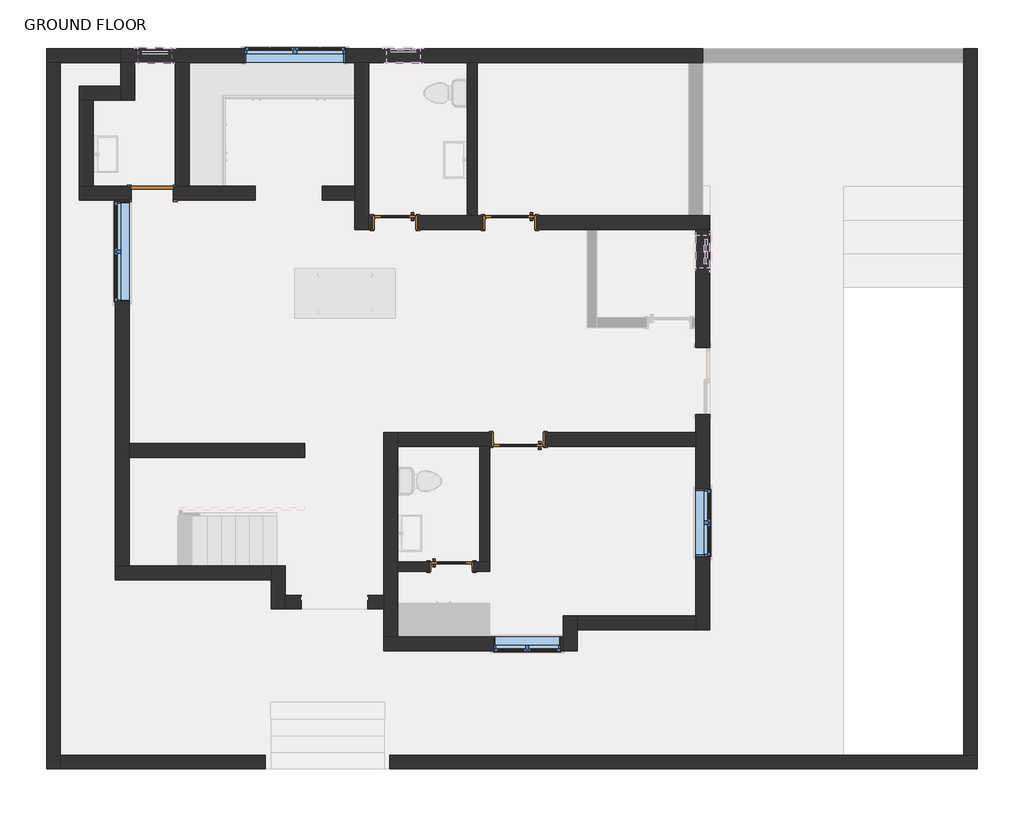
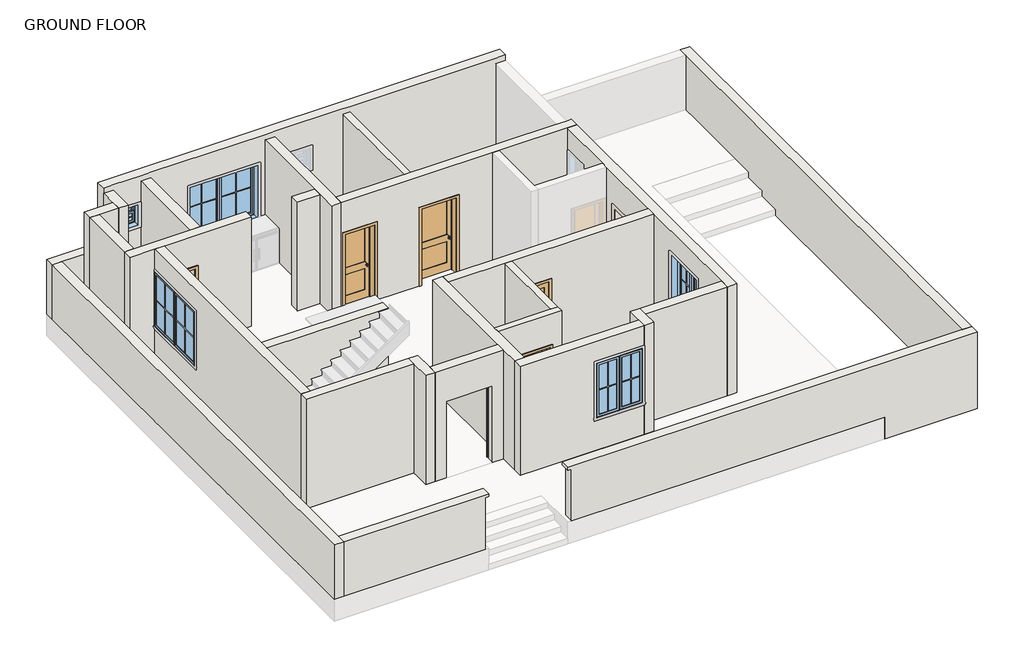
# One storey, part 1 of 2: 28 walls, 5 doors, 5 windows.
"""IFC4 building model written with IfcOpenShell, lengths in millimetres."""

from ifc_helpers import new_model, si_unit, frame, origin, origin_with_axes, place, context, project, spatial, polyline, outline, extrude, faceted_brep, transform, mapped, element, save
from components import door_e3d10b2c, door_ff2e0a99, door_acb80719, door_97a41ff7, door_bfeef022, window_casement_double_4_a93ed6b4, window_casement_double_6_75db422f, window_double_hung_2_d0105baa

model = new_model("IFC4")

# Units and contexts
model_context = context("Model", 3, world=origin())
ifc_project = project(units=[si_unit("LENGTHUNIT", "METRE", prefix="MILLI")], contexts=[model_context])

# Site, building, storey
site = spatial("IfcSite", under=ifc_project)
building = spatial("IfcBuilding", under=site)
storey = spatial("IfcBuildingStorey", under=building, Name="GROUND FLOOR", Elevation=0.0)

# Doors
placement = place(None, origin())
door_shape = door_e3d10b2c(model_context)
element("IfcDoor", 1, ObjectType="Door-Interior-Single-2_Panel-Wood : 2'6\"", at=placement, inside=storey, context=model_context, shape_type="MappedRepresentation", body=[
    mapped(door_shape, transform((-3580.8201068, 2930.9627014, 0.0), x_axis=(-1.0, 0.0, 0.0), y_axis=(0.0, -1.0, 0.0), z_axis=(0.0, 0.0, 1.0))),
])
door_2_shape = door_ff2e0a99(model_context)
element("IfcDoor", 2, ObjectType="Door-Interior-Single-2_Panel-Wood : 2'6\"", at=placement, inside=storey, context=model_context, shape_type="MappedRepresentation", body=[
    mapped(door_2_shape, transform((-2552.1201068, -3355.5372986, 0.0), x_axis=(1.0, 0.0, 0.0), y_axis=(0.0, 1.0, 0.0), z_axis=(0.0, 0.0, 1.0))),
])
door_3_shape = door_acb80719(model_context)
element("IfcDoor", 3, ObjectType="Door-Interior-Single-2_Panel-Wood : 36\" x 84\"", at=placement, inside=storey, context=model_context, shape_type="MappedRepresentation", body=[
    mapped(door_3_shape, transform((-1485.3201068, 2930.9627014, 0.0), x_axis=(-1.0, 0.0, 0.0), y_axis=(0.0, -1.0, 0.0), z_axis=(0.0, 0.0, 1.0))),
])
door_4_shape = door_97a41ff7(model_context)
element("IfcDoor", 4, ObjectType="Door-Interior-Single-2_Panel-Wood : 36\" x 84\"", at=placement, inside=storey, context=model_context, shape_type="MappedRepresentation", body=[
    mapped(door_4_shape, transform((-1332.9201068, -1037.7872986, 0.0), x_axis=(-1.0, 0.0, 0.0), y_axis=(0.0, -1.0, 0.0), z_axis=(0.0, 0.0, 1.0))),
])
door_5_shape = door_bfeef022(model_context)
element("IfcDoor", 5, ObjectType="Single-Flush : 2'6\"", at=placement, inside=storey, context=model_context, shape_type="MappedRepresentation", body=[
    mapped(door_5_shape, transform((-8013.1201068, 3461.1877014, 0.0), x_axis=(1.0, 0.0, 0.0), y_axis=(0.0, 1.0, 0.0), z_axis=(0.0, 0.0, 1.0))),
])

# Walls
element("IfcWall", 6, at=placement, inside=storey, context=model_context, shape_type="Brep", body=[
    faceted_brep([(-9346.6201068, 5162.9877014, 0.0), (-9092.6201068, 5162.9877014, 0.0), (-8584.6201068, 5162.9877014, 0.0), (-8584.6201068, 5162.9877014, 3048.0), (-9092.6201068, 5162.9877014, 3048.0), (-9346.6201068, 5162.9877014, 3048.0), (-8584.6201068, 5416.9877014, 0.0), (-9346.6201068, 5416.9877014, 0.0), (-9346.6201068, 5416.9877014, 3048.0), (-8584.6201068, 5416.9877014, 3048.0)], [[[0, 1, 2, 3, 4, 5]], [[6, 7, 8, 9]], [[2, 1, 0, 7, 6]], [[2, 6, 9, 3]], [[7, 0, 5, 8]], [[5, 4, 3, 9, 8]]]),
])
element("IfcWall", 7, at=placement, inside=storey, context=model_context, shape_type="Brep", body=[
    faceted_brep([(-8330.6201068, 5162.9877014, 0.0), (-8330.6201068, 5848.7877014, 0.0), (-8330.6201068, 5848.7877014, 3048.0), (-8330.6201068, 5162.9877014, 3048.0), (-8584.6201068, 5848.7877014, 0.0), (-8584.6201068, 5416.9877014, 0.0), (-8584.6201068, 5162.9877014, 0.0), (-8584.6201068, 5162.9877014, 3048.0), (-8584.6201068, 5416.9877014, 3048.0), (-8584.6201068, 5848.7877014, 3048.0)], [[[0, 1, 2, 3]], [[4, 5, 6, 7, 8, 9]], [[1, 0, 6, 5, 4]], [[6, 0, 3, 7]], [[1, 4, 9, 2]], [[3, 2, 9, 8, 7]]]),
])
element("IfcWall", 8, at=placement, inside=storey, context=model_context, shape_type="Brep", body=[
    faceted_brep([(-8584.6201068, 5848.7877014, 3200.4), (-8584.6201068, 5848.7877014, 1524.0), (-8584.6201068, 5848.7877014, 0.0), (-8330.6201068, 5848.7877014, 0.0), (-7594.0201068, 5848.7877014, 0.0), (-7340.0201068, 5848.7877014, 0.0), (-4317.4201068, 5848.7877014, 0.0), (-4063.4201068, 5848.7877014, 0.0), (-2260.0201068, 5848.7877014, 0.0), (-2082.2201068, 5848.7877014, 0.0), (1778.5798932, 5848.7877014, 0.0), (2032.5798932, 5848.7877014, 0.0), (2032.5798932, 5848.7877014, 1524.0), (2032.5798932, 5848.7877014, 3200.4), (1778.5798932, 5848.7877014, 3200.4), (-2082.2201068, 5848.7877014, 3200.4), (-2260.0201068, 5848.7877014, 3200.4), (-4063.4201068, 5848.7877014, 3200.4), (-4317.4201068, 5848.7877014, 3200.4), (-7340.0201068, 5848.7877014, 3200.4), (-7594.0201068, 5848.7877014, 3200.4), (-8330.6201068, 5848.7877014, 3200.4), (-4495.2201068, 5848.7877014, 2438.4), (-4495.2201068, 5848.7877014, 914.4), (-6324.0201068, 5848.7877014, 914.4), (-6324.0201068, 5848.7877014, 2438.4), (-3733.2201068, 5848.7877014, 2438.4), (-3123.6201068, 5848.7877014, 2438.4), (-3123.6201068, 5848.7877014, 1828.8), (-3733.2201068, 5848.7877014, 1828.8), (-8267.1201068, 5848.7877014, 2438.4), (-7657.5201068, 5848.7877014, 2438.4), (-7657.5201068, 5848.7877014, 1828.8), (-8267.1201068, 5848.7877014, 1828.8), (-8584.6201068, 6102.7877014, 0.0), (-8584.6201068, 6102.7877014, 1524.0), (-8584.6201068, 6102.7877014, 3200.4), (2032.5798932, 6102.7877014, 3200.4), (2032.5798932, 6102.7877014, 1524.0), (2032.5798932, 6102.7877014, 0.0), (-4495.2201068, 6102.7877014, 2438.4), (-6324.0201068, 6102.7877014, 2438.4), (-6324.0201068, 6102.7877014, 914.4), (-4495.2201068, 6102.7877014, 914.4), (-3733.2201068, 6102.7877014, 2438.4), (-3733.2201068, 6102.7877014, 1828.8), (-3123.6201068, 6102.7877014, 1828.8), (-3123.6201068, 6102.7877014, 2438.4), (-8267.1201068, 6102.7877014, 2438.4), (-8267.1201068, 6102.7877014, 1828.8), (-7657.5201068, 6102.7877014, 1828.8), (-7657.5201068, 6102.7877014, 2438.4)], [[[0, 1, 2, 3, 4, 5, 6, 7, 8, 9, 10, 11, 12, 13, 14, 15, 16, 17, 18, 19, 20, 21], [22, 23, 24, 25], [26, 27, 28, 29], [30, 31, 32, 33]], [[34, 35, 36, 37, 38, 39], [40, 41, 42, 43], [44, 45, 46, 47], [48, 49, 50, 51]], [[11, 10, 9, 8, 7, 6, 5, 4, 3, 2, 34, 39]], [[0, 21, 20, 19, 18, 17, 16, 15, 14, 13, 37, 36]], [[23, 22, 40, 43]], [[24, 23, 43, 42]], [[25, 24, 42, 41]], [[22, 25, 41, 40]], [[45, 44, 26, 29]], [[46, 45, 29, 28]], [[47, 46, 28, 27]], [[44, 47, 27, 26]], [[49, 48, 30, 33]], [[50, 49, 33, 32]], [[51, 50, 32, 31]], [[48, 51, 31, 30]], [[0, 36, 35, 34, 2, 1]], [[11, 39, 38, 37, 13, 12]]]),
])
element("IfcWall", 9, at=placement, inside=storey, context=model_context, shape_type="SweptSolid", body=[
    extrude(outline(polyline([(-7594.0201068, 3588.1877014), (-7594.0201068, 5848.7877014), (-7340.0201068, 5848.7877014), (-7340.0201068, 3588.1877014), (-7594.0201068, 3588.1877014)])), origin_with_axes(), (0.0, 0.0, 1.0), 3048.0),
])
element("IfcWall", 10, at=placement, inside=storey, context=model_context, shape_type="Brep", body=[
    faceted_brep([(1905.5798932, 641.7877014, 0.0), (1905.5798932, 641.7877014, 2133.6), (1905.5798932, -577.4122986, 2133.6), (1905.5798932, -577.4122986, 0.0), (1905.5798932, -907.6122986, 0.0), (1905.5798932, -1161.6122986, 0.0), (1905.5798932, -4260.4122986, 0.0), (1905.5798932, -4514.4122986, 0.0), (1905.5798932, -4514.4122986, 3048.0), (1905.5798932, -4260.4122986, 3048.0), (1905.5798932, -1161.6122986, 3048.0), (1905.5798932, -907.6122986, 3048.0), (1905.5798932, 1010.0877014, 3048.0), (1905.5798932, 1187.8877014, 3048.0), (1905.5798932, 2800.7877014, 3048.0), (1905.5798932, 2800.7877014, 0.0), (1905.5798932, 1187.8877014, 0.0), (1905.5798932, 1010.0877014, 0.0), (1905.5798932, -3168.2122986, 2438.4), (1905.5798932, -3168.2122986, 914.4), (1905.5798932, -1949.0122986, 914.4), (1905.5798932, -1949.0122986, 2438.4), (1905.5798932, 2089.5877014, 1828.8), (1905.5798932, 2699.1877014, 1828.8), (1905.5798932, 2699.1877014, 2438.4), (1905.5798932, 2089.5877014, 2438.4), (2159.5798932, 641.7877014, 2133.6), (2159.5798932, 641.7877014, 0.0), (2159.5798932, 2800.7877014, 0.0), (2159.5798932, 2800.7877014, 3048.0), (2159.5798932, -4514.4122986, 3048.0), (2159.5798932, -4514.4122986, 0.0), (2159.5798932, -577.4122986, 0.0), (2159.5798932, -577.4122986, 2133.6), (2159.5798932, -3168.2122986, 914.4), (2159.5798932, -3168.2122986, 2438.4), (2159.5798932, -1949.0122986, 2438.4), (2159.5798932, -1949.0122986, 914.4), (2159.5798932, 2699.1877014, 1828.8), (2159.5798932, 2089.5877014, 1828.8), (2159.5798932, 2089.5877014, 2438.4), (2159.5798932, 2699.1877014, 2438.4)], [[[0, 1, 2, 3, 4, 5, 6, 7, 8, 9, 10, 11, 12, 13, 14, 15, 16, 17], [18, 19, 20, 21], [22, 23, 24, 25]], [[26, 27, 28, 29, 30, 31, 32, 33], [34, 35, 36, 37], [38, 39, 40, 41]], [[15, 28, 27, 0, 17, 16]], [[31, 7, 6, 5, 4, 3, 32]], [[28, 15, 14, 29]], [[7, 31, 30, 8]], [[19, 18, 35, 34]], [[20, 19, 34, 37]], [[21, 20, 37, 36]], [[18, 21, 36, 35]], [[22, 39, 38, 23]], [[39, 22, 25, 40]], [[40, 25, 24, 41]], [[23, 38, 41, 24]], [[14, 13, 12, 11, 10, 9, 8, 30, 29]], [[27, 26, 1, 0]], [[33, 32, 3, 2]], [[26, 33, 2, 1]]]),
])
element("IfcWall", 11, at=placement, inside=storey, context=model_context, shape_type="SweptSolid", body=[
    extrude(outline(polyline([(-253.4201068, -4260.4122986), (1905.5798932, -4260.4122986), (1905.5798932, -4514.4122986), (-253.4201068, -4514.4122986), (-253.4201068, -4260.4122986)])), origin_with_axes(), (0.0, 0.0, 1.0), 3048.0),
])
element("IfcWall", 12, at=placement, inside=storey, context=model_context, shape_type="Brep", body=[
    faceted_brep([(-253.4201068, -4895.4122986, 0.0), (-253.4201068, -4514.4122986, 0.0), (-253.4201068, -4260.4122986, 0.0), (-253.4201068, -4260.4122986, 3048.0), (-253.4201068, -4514.4122986, 3048.0), (-253.4201068, -4895.4122986, 3048.0), (-507.4201068, -4260.4122986, 0.0), (-507.4201068, -4641.4122986, 0.0), (-507.4201068, -4895.4122986, 0.0), (-507.4201068, -4895.4122986, 3048.0), (-507.4201068, -4641.4122986, 3048.0), (-507.4201068, -4260.4122986, 3048.0)], [[[0, 1, 2, 3, 4, 5]], [[6, 7, 8, 9, 10, 11]], [[2, 1, 0, 8, 7, 6]], [[2, 6, 11, 3]], [[8, 0, 5, 9]], [[4, 3, 11, 10, 9, 5]]]),
])
element("IfcWall", 13, at=placement, inside=storey, context=model_context, shape_type="Brep", body=[
    faceted_brep([(-507.4201068, -4641.4122986, 0.0), (-3530.0201068, -4641.4122986, 0.0), (-3784.0201068, -4641.4122986, 0.0), (-3784.0201068, -4641.4122986, 3048.0), (-3530.0201068, -4641.4122986, 3048.0), (-507.4201068, -4641.4122986, 3048.0), (-1777.4201068, -4641.4122986, 2438.4), (-1777.4201068, -4641.4122986, 914.4), (-558.2201068, -4641.4122986, 914.4), (-558.2201068, -4641.4122986, 2438.4), (-3784.0201068, -4895.4122986, 0.0), (-507.4201068, -4895.4122986, 0.0), (-507.4201068, -4895.4122986, 3048.0), (-3784.0201068, -4895.4122986, 3048.0), (-1777.4201068, -4895.4122986, 914.4), (-1777.4201068, -4895.4122986, 2438.4), (-558.2201068, -4895.4122986, 2438.4), (-558.2201068, -4895.4122986, 914.4)], [[[0, 1, 2, 3, 4, 5], [6, 7, 8, 9]], [[10, 11, 12, 13], [14, 15, 16, 17]], [[2, 1, 0, 11, 10]], [[11, 0, 5, 12]], [[2, 10, 13, 3]], [[7, 6, 15, 14]], [[8, 7, 14, 17]], [[9, 8, 17, 16]], [[6, 9, 16, 15]], [[5, 4, 3, 13, 12]]]),
])
element("IfcWall", 14, at=placement, inside=storey, context=model_context, shape_type="Brep", body=[
    faceted_brep([(-3530.0201068, -4641.4122986, 0.0), (-3530.0201068, -3447.6122986, 0.0), (-3530.0201068, -3269.8122986, 0.0), (-3530.0201068, -1161.6122986, 0.0), (-3530.0201068, -907.6122986, 0.0), (-3530.0201068, -907.6122986, 3048.0), (-3530.0201068, -1161.6122986, 3048.0), (-3530.0201068, -3269.8122986, 3048.0), (-3530.0201068, -3447.6122986, 3048.0), (-3530.0201068, -4641.4122986, 3048.0), (-3784.0201068, -907.6122986, 0.0), (-3784.0201068, -3879.4122986, 0.0), (-3784.0201068, -4133.4122986, 0.0), (-3784.0201068, -4641.4122986, 0.0), (-3784.0201068, -4641.4122986, 3048.0), (-3784.0201068, -4133.4122986, 3048.0), (-3784.0201068, -907.6122986, 3048.0)], [[[0, 1, 2, 3, 4, 5, 6, 7, 8, 9]], [[10, 11, 12, 13, 14, 15, 16]], [[4, 3, 2, 1, 0, 13, 12, 11, 10]], [[13, 0, 9, 14]], [[4, 10, 16, 5]], [[9, 8, 7, 6, 5, 16, 15, 14]]]),
])
element("IfcWall", 15, at=placement, inside=storey, context=model_context, shape_type="Brep", body=[
    faceted_brep([(-3530.0201068, -1161.6122986, 0.0), (-2031.4201068, -1161.6122986, 0.0), (-1853.6201068, -1161.6122986, 0.0), (-1815.5201068, -1161.6122986, 0.0), (-1815.5201068, -1161.6122986, 2159.0), (-850.3201068, -1161.6122986, 2159.0), (-850.3201068, -1161.6122986, 0.0), (1905.5798932, -1161.6122986, 0.0), (1905.5798932, -1161.6122986, 3048.0), (-3530.0201068, -1161.6122986, 3048.0), (-1815.5201068, -907.6122986, 0.0), (-3530.0201068, -907.6122986, 0.0), (-3530.0201068, -907.6122986, 3048.0), (1905.5798932, -907.6122986, 3048.0), (1905.5798932, -907.6122986, 0.0), (-850.3201068, -907.6122986, 0.0), (-850.3201068, -907.6122986, 2159.0), (-1815.5201068, -907.6122986, 2159.0)], [[[0, 1, 2, 3, 4, 5, 6, 7, 8, 9]], [[10, 11, 12, 13, 14, 15, 16, 17]], [[0, 11, 10, 3, 2, 1]], [[14, 7, 6, 15]], [[11, 0, 9, 12]], [[7, 14, 13, 8]], [[17, 4, 3, 10]], [[4, 17, 16, 5]], [[5, 16, 15, 6]], [[9, 8, 13, 12]]]),
])
element("IfcWall", 16, at=placement, inside=storey, context=model_context, shape_type="Brep", body=[
    faceted_brep([(-5295.3201068, -3879.4122986, 0.0), (-5587.4201068, -3879.4122986, 0.0), (-5587.4201068, -3879.4122986, 3048.0), (-3784.0201068, -3879.4122986, 3048.0), (-3784.0201068, -3879.4122986, 0.0), (-4076.1201068, -3879.4122986, 0.0), (-4076.1201068, -3879.4122986, 2133.6), (-5295.3201068, -3879.4122986, 2133.6), (-5587.4201068, -4133.4122986, 0.0), (-5295.3201068, -4133.4122986, 0.0), (-5295.3201068, -4133.4122986, 2133.6), (-4076.1201068, -4133.4122986, 2133.6), (-4076.1201068, -4133.4122986, 0.0), (-3784.0201068, -4133.4122986, 0.0), (-3784.0201068, -4133.4122986, 3048.0), (-5587.4201068, -4133.4122986, 3048.0), (-4076.1201068, -3976.4122986, 0.0), (-4061.1201068, -3976.4122986, 0.0), (-4061.1201068, -3899.4122986, 0.0), (-4076.1201068, -3899.4122986, 0.0), (-5295.3201068, -3899.4122986, 0.0), (-5310.3201068, -3899.4122986, 0.0), (-5310.3201068, -3976.4122986, 0.0), (-5295.3201068, -3976.4122986, 0.0), (-5295.3201068, -3899.4122986, 2133.6), (-4076.1201068, -3899.4122986, 2133.6), (-4061.1201068, -3899.4122986, 2148.6), (-5310.3201068, -3899.4122986, 2148.6), (-5310.3201068, -3976.4122986, 2148.6), (-4061.1201068, -3976.4122986, 2148.6), (-4076.1201068, -3976.4122986, 2133.6), (-5295.3201068, -3976.4122986, 2133.6)], [[[0, 1, 2, 3, 4, 5, 6, 7]], [[8, 9, 10, 11, 12, 13, 14, 15]], [[4, 13, 12, 16, 17, 18, 19, 5]], [[8, 1, 0, 20, 21, 22, 23, 9]], [[13, 4, 3, 14]], [[1, 8, 15, 2]], [[24, 20, 0, 7]], [[19, 25, 6, 5]], [[25, 24, 7, 6]], [[20, 24, 25, 19, 18, 26, 27, 21]], [[21, 27, 28, 22]], [[22, 28, 29, 17, 16, 30, 31, 23]], [[27, 26, 29, 28]], [[26, 18, 17, 29]], [[23, 31, 10, 9]], [[30, 16, 12, 11]], [[31, 30, 11, 10]], [[3, 2, 15, 14]]]),
])
element("IfcWall", 17, at=placement, inside=storey, context=model_context, shape_type="Brep", body=[
    faceted_brep([(-5587.4201068, -4133.4122986, 0.0), (-5587.4201068, -3879.4122986, 0.0), (-5587.4201068, -3346.0122986, 0.0), (-5587.4201068, -3346.0122986, 3048.0), (-5587.4201068, -3879.4122986, 3048.0), (-5587.4201068, -4133.4122986, 3048.0), (-5841.4201068, -3346.0122986, 0.0), (-5841.4201068, -3600.0122986, 0.0), (-5841.4201068, -4133.4122986, 0.0), (-5841.4201068, -4133.4122986, 3048.0), (-5841.4201068, -3600.0122986, 3048.0), (-5841.4201068, -3346.0122986, 3048.0)], [[[0, 1, 2, 3, 4, 5]], [[6, 7, 8, 9, 10, 11]], [[2, 1, 0, 8, 7, 6]], [[8, 0, 5, 9]], [[2, 6, 11, 3]], [[5, 4, 3, 11, 10, 9]]]),
])
element("IfcWall", 18, at=placement, inside=storey, context=model_context, shape_type="Brep", body=[
    faceted_brep([(-5841.4201068, -3346.0122986, 0.0), (-8432.2201068, -3346.0122986, 0.0), (-8686.2201068, -3346.0122986, 0.0), (-8686.2201068, -3346.0122986, 3048.0), (-8432.2201068, -3346.0122986, 3048.0), (-5841.4201068, -3346.0122986, 3048.0), (-8686.2201068, -3600.0122986, 0.0), (-5841.4201068, -3600.0122986, 0.0), (-5841.4201068, -3600.0122986, 3048.0), (-8686.2201068, -3600.0122986, 3048.0)], [[[0, 1, 2, 3, 4, 5]], [[6, 7, 8, 9]], [[2, 1, 0, 7, 6]], [[7, 0, 5, 8]], [[2, 6, 9, 3]], [[5, 4, 3, 9, 8]]]),
])
element("IfcWall", 19, at=placement, inside=storey, context=model_context, shape_type="Brep", body=[
    faceted_brep([(-8432.2201068, -3346.0122986, 0.0), (-8432.2201068, -1364.8122986, 0.0), (-8432.2201068, -1110.8122986, 0.0), (-8432.2201068, 3334.1877014, 0.0), (-8432.2201068, 3334.1877014, 3048.0), (-8432.2201068, -1364.8122986, 3048.0), (-8432.2201068, -3346.0122986, 3048.0), (-8432.2201068, 3308.7877014, 2438.4), (-8432.2201068, 3308.7877014, 914.4), (-8432.2201068, 1479.9877014, 914.4), (-8432.2201068, 1479.9877014, 2438.4), (-8686.2201068, 3334.1877014, 0.0), (-8686.2201068, -3346.0122986, 0.0), (-8686.2201068, -3346.0122986, 3048.0), (-8686.2201068, 3334.1877014, 3048.0), (-8686.2201068, 3308.7877014, 914.4), (-8686.2201068, 3308.7877014, 2438.4), (-8686.2201068, 1479.9877014, 2438.4), (-8686.2201068, 1479.9877014, 914.4)], [[[0, 1, 2, 3, 4, 5, 6], [7, 8, 9, 10]], [[11, 12, 13, 14], [15, 16, 17, 18]], [[3, 2, 1, 0, 12, 11]], [[12, 0, 6, 13]], [[3, 11, 14, 4]], [[8, 7, 16, 15]], [[9, 8, 15, 18]], [[10, 9, 18, 17]], [[7, 10, 17, 16]], [[6, 5, 4, 14, 13]]]),
])
element("IfcWall", 20, at=placement, inside=storey, context=model_context, shape_type="Brep", body=[
    faceted_brep([(-7632.1201068, 3588.1877014, 0.0), (-7632.1201068, 3588.1877014, 2133.6), (-8394.1201068, 3588.1877014, 2133.6), (-8394.1201068, 3588.1877014, 0.0), (-9092.6201068, 3588.1877014, 0.0), (-9346.6201068, 3588.1877014, 0.0), (-9346.6201068, 3588.1877014, 3048.0), (-6133.5201068, 3588.1877014, 3048.0), (-6133.5201068, 3588.1877014, 0.0), (-7340.0201068, 3588.1877014, 0.0), (-7594.0201068, 3588.1877014, 0.0), (-7632.1201068, 3334.1877014, 2133.6), (-7632.1201068, 3334.1877014, 0.0), (-6133.5201068, 3334.1877014, 0.0), (-6133.5201068, 3334.1877014, 3048.0), (-8432.2201068, 3334.1877014, 3048.0), (-8686.2201068, 3334.1877014, 3048.0), (-9346.6201068, 3334.1877014, 3048.0), (-9346.6201068, 3334.1877014, 0.0), (-8686.2201068, 3334.1877014, 0.0), (-8432.2201068, 3334.1877014, 0.0), (-8394.1201068, 3334.1877014, 0.0), (-8394.1201068, 3334.1877014, 2133.6)], [[[0, 1, 2, 3, 4, 5, 6, 7, 8, 9, 10]], [[11, 12, 13, 14, 15, 16, 17, 18, 19, 20, 21, 22]], [[8, 13, 12, 0, 10, 9]], [[18, 5, 4, 3, 21, 20, 19]], [[13, 8, 7, 14]], [[5, 18, 17, 6]], [[1, 0, 12, 11]], [[2, 1, 11, 22]], [[3, 2, 22, 21]], [[7, 6, 17, 16, 15, 14]]]),
])
element("IfcWall", 21, at=placement, inside=storey, context=model_context, shape_type="SweptSolid", body=[
    extrude(outline(polyline([(-9092.6201068, 5162.9877014), (-9092.6201068, 3588.1877014), (-9346.6201068, 3588.1877014), (-9346.6201068, 5162.9877014), (-9092.6201068, 5162.9877014)])), origin_with_axes(), (0.0, 0.0, 1.0), 3048.0),
])
element("IfcWall", 22, at=placement, inside=storey, context=model_context, shape_type="Brep", body=[
    faceted_brep([(-4063.4201068, 2800.7877014, 0.0), (-4063.4201068, 3054.7877014, 0.0), (-4063.4201068, 5848.7877014, 0.0), (-4063.4201068, 5848.7877014, 3048.0), (-4063.4201068, 3054.7877014, 3048.0), (-4063.4201068, 2800.7877014, 3048.0), (-4317.4201068, 5848.7877014, 0.0), (-4317.4201068, 3588.1877014, 0.0), (-4317.4201068, 3334.1877014, 0.0), (-4317.4201068, 2800.7877014, 0.0), (-4317.4201068, 2800.7877014, 3048.0), (-4317.4201068, 5848.7877014, 3048.0)], [[[0, 1, 2, 3, 4, 5]], [[6, 7, 8, 9, 10, 11]], [[2, 1, 0, 9, 8, 7, 6]], [[2, 6, 11, 3]], [[9, 0, 5, 10]], [[5, 4, 3, 11, 10]]]),
])
element("IfcWall", 23, at=placement, inside=storey, context=model_context, shape_type="Brep", body=[
    faceted_brep([(-1002.7201068, 2800.7877014, 0.0), (-75.6201068, 2800.7877014, 0.0), (102.1798932, 2800.7877014, 0.0), (1905.5798932, 2800.7877014, 0.0), (2159.5798932, 2800.7877014, 0.0), (2159.5798932, 2800.7877014, 3048.0), (-4063.4201068, 2800.7877014, 3048.0), (-4063.4201068, 2800.7877014, 0.0), (-3987.2201068, 2800.7877014, 0.0), (-3987.2201068, 2800.7877014, 2159.0), (-3174.4201068, 2800.7877014, 2159.0), (-3174.4201068, 2800.7877014, 0.0), (-1967.9201068, 2800.7877014, 0.0), (-1967.9201068, 2800.7877014, 2159.0), (-1002.7201068, 2800.7877014, 2159.0), (2159.5798932, 3054.7877014, 0.0), (2032.5798932, 3054.7877014, 0.0), (1778.5798932, 3054.7877014, 0.0), (-1002.7201068, 3054.7877014, 0.0), (-1002.7201068, 3054.7877014, 2159.0), (-1967.9201068, 3054.7877014, 2159.0), (-1967.9201068, 3054.7877014, 0.0), (-2082.2201068, 3054.7877014, 0.0), (-2260.0201068, 3054.7877014, 0.0), (-3174.4201068, 3054.7877014, 0.0), (-3174.4201068, 3054.7877014, 2159.0), (-3987.2201068, 3054.7877014, 2159.0), (-3987.2201068, 3054.7877014, 0.0), (-4063.4201068, 3054.7877014, 0.0), (-4063.4201068, 3054.7877014, 3048.0), (1778.5798932, 3054.7877014, 3048.0), (2032.5798932, 3054.7877014, 3048.0), (2159.5798932, 3054.7877014, 3048.0)], [[[0, 1, 2, 3, 4, 5, 6, 7, 8, 9, 10, 11, 12, 13, 14]], [[15, 16, 17, 18, 19, 20, 21, 22, 23, 24, 25, 26, 27, 28, 29, 30, 31, 32]], [[15, 4, 3, 2, 1, 0, 18, 17, 16]], [[21, 12, 11, 24, 23, 22]], [[8, 7, 28, 27]], [[4, 15, 32, 5]], [[20, 13, 12, 21]], [[13, 20, 19, 14]], [[14, 19, 18, 0]], [[26, 9, 8, 27]], [[9, 26, 25, 10]], [[10, 25, 24, 11]], [[28, 7, 6, 29]], [[6, 5, 32, 31, 30, 29]]]),
])
element("IfcWall", 24, at=placement, inside=storey, context=model_context, shape_type="SweptSolid", body=[
    extrude(outline(polyline([(-4317.4201068, 3334.1877014), (-4914.3201068, 3334.1877014), (-4914.3201068, 3588.1877014), (-4317.4201068, 3588.1877014), (-4317.4201068, 3334.1877014)])), origin_with_axes(), (0.0, 0.0, 1.0), 3048.0),
])
element("IfcWall", 25, at=placement, inside=storey, context=model_context, shape_type="Brep", body=[
    faceted_brep([(-8584.6201068, 6102.7877014, 0.0), (-9943.5201068, 6102.7877014, 0.0), (-9943.5201068, 6102.7877014, 1524.0), (-8584.6201068, 6102.7877014, 1524.0), (-8584.6201068, 5848.7877014, 0.0), (-8584.6201068, 5848.7877014, 1524.0), (-9689.5201068, 5848.7877014, 1524.0), (-9943.5201068, 5848.7877014, 1524.0), (-9943.5201068, 5848.7877014, 0.0), (-9689.5201068, 5848.7877014, 0.0)], [[[0, 1, 2, 3]], [[4, 5, 6, 7, 8, 9]], [[1, 0, 4, 9, 8]], [[3, 2, 7, 6, 5]], [[0, 3, 5, 4]], [[2, 1, 8, 7]]]),
])
element("IfcWall", 26, at=placement, inside=storey, context=model_context, shape_type="Brep", body=[
    faceted_brep([(-9943.5201068, 5848.7877014, 0.0), (-9943.5201068, -7054.4122986, 0.0), (-9943.5201068, -7054.4122986, 1524.0), (-9943.5201068, 5848.7877014, 1524.0), (-9689.5201068, 5848.7877014, 0.0), (-9689.5201068, 5848.7877014, 1524.0), (-9689.5201068, -6800.4122986, 1524.0), (-9689.5201068, -7054.4122986, 1524.0), (-9689.5201068, -7054.4122986, 0.0), (-9689.5201068, -6800.4122986, 0.0)], [[[0, 1, 2, 3]], [[4, 5, 6, 7, 8, 9]], [[1, 0, 4, 9, 8]], [[3, 2, 7, 6, 5]], [[0, 3, 5, 4]], [[2, 1, 8, 7]]]),
])
element("IfcWall", 27, at=placement, inside=storey, context=model_context, shape_type="Brep", body=[
    faceted_brep([(7049.0798932, 6102.7877014, 1524.0), (7049.0798932, -6800.4122986, 1524.0), (7049.0798932, -6800.4122986, -457.2), (7049.0798932, 1746.6877014, -457.2), (7049.0798932, 1746.6877014, -304.8), (7049.0798932, 2356.2877014, -304.8), (7049.0798932, 2356.2877014, -152.4), (7049.0798932, 2972.2377014, -152.4), (7049.0798932, 2972.2377014, 0.0), (7049.0798932, 3588.1877014, 0.0), (7049.0798932, 6102.7877014, 0.0), (6795.0798932, -6800.4122986, 1524.0), (6795.0798932, 5848.7877014, 1524.0), (6795.0798932, 6102.7877014, 1524.0), (6795.0798932, 6102.7877014, 0.0), (6795.0798932, 5848.7877014, 0.0), (6795.0798932, 2972.2377014, 0.0), (6795.0798932, 2972.2377014, -152.4), (6795.0798932, 2356.2877014, -152.4), (6795.0798932, 2356.2877014, -304.8), (6795.0798932, 1746.6877014, -304.8), (6795.0798932, 1746.6877014, -457.2), (6795.0798932, -6800.4122986, -457.2)], [[[0, 1, 2, 3, 4, 5, 6, 7, 8, 9, 10]], [[11, 12, 13, 14, 15, 16, 17, 18, 19, 20, 21, 22]], [[2, 22, 21, 3]], [[1, 0, 13, 12, 11]], [[2, 1, 11, 22]], [[13, 0, 10, 14]], [[14, 10, 9, 8, 16, 15]], [[16, 8, 7, 17]], [[6, 18, 17, 7]], [[18, 6, 5, 19]], [[4, 20, 19, 5]], [[20, 4, 3, 21]]]),
])
element("IfcWall", 28, at=placement, inside=storey, context=model_context, shape_type="SweptSolid", body=[
    extrude(outline(polyline([(1524.0, -5854.1201068), (1524.0, -9689.5201068), (0.0, -9689.5201068), (0.0, -5948.2201068), (1442.4, -5948.2201068), (1442.4, -5854.1201068), (1524.0, -5854.1201068)])), frame((0.0, -7054.4122986, 0.0), z_axis=(0.0, 1.0, 0.0), x_axis=(0.0, 0.0, 1.0)), (0.0, 0.0, 1.0), 254.0),
])
element("IfcWall", 29, at=placement, inside=storey, context=model_context, shape_type="Brep", body=[
    faceted_brep([(7049.0798932, -7054.4122986, 1524.0), (-3771.3201068, -7054.4122986, 1524.0), (-3771.3201068, -7054.4122986, 1442.4), (-3677.2201068, -7054.4122986, 1442.4), (-3677.2201068, -7054.4122986, 0.0), (4597.9798932, -7054.4122986, 0.0), (4597.9798932, -7054.4122986, -609.6), (7049.0798932, -7054.4122986, -609.6), (-3771.3201068, -6800.4122986, 1524.0), (6795.0798932, -6800.4122986, 1524.0), (7049.0798932, -6800.4122986, 1524.0), (7049.0798932, -6800.4122986, -457.2), (7049.0798932, -6800.4122986, -609.6), (4597.9798932, -6800.4122986, -609.6), (4597.9798932, -6800.4122986, 0.0), (-3677.2201068, -6800.4122986, 0.0), (-3677.2201068, -6800.4122986, 1442.4), (-3771.3201068, -6800.4122986, 1442.4)], [[[0, 1, 2, 3, 4, 5, 6, 7]], [[8, 9, 10, 11, 12, 13, 14, 15, 16, 17]], [[12, 7, 6, 13]], [[1, 0, 10, 9, 8]], [[1, 8, 17, 2]], [[0, 7, 12, 11, 10]], [[14, 5, 4, 15]], [[5, 14, 13, 6]], [[3, 16, 15, 4]], [[16, 3, 2, 17]]]),
])
element("IfcWall", 30, at=placement, inside=storey, context=model_context, shape_type="SweptSolid", body=[
    extrude(outline(polyline([(-5231.8201068, -1364.8122986), (-8432.2201068, -1364.8122986), (-8432.2201068, -1110.8122986), (-5231.8201068, -1110.8122986), (-5231.8201068, -1364.8122986)])), origin_with_axes(), (0.0, 0.0, 1.0), 3048.0),
])
element("IfcWall", 31, ObjectType="6\" WALL", at=placement, inside=storey, context=model_context, shape_type="Brep", body=[
    faceted_brep([(-1853.6201068, -3269.8122986, 0.0), (-2031.4201068, -3269.8122986, 0.0), (-2145.7201068, -3269.8122986, 0.0), (-2145.7201068, -3269.8122986, 2159.0), (-2958.5201068, -3269.8122986, 2159.0), (-2958.5201068, -3269.8122986, 0.0), (-3530.0201068, -3269.8122986, 0.0), (-3530.0201068, -3269.8122986, 3048.0), (-2031.4201068, -3269.8122986, 3048.0), (-1853.6201068, -3269.8122986, 3048.0), (-2145.7201068, -3447.6122986, 0.0), (-1853.6201068, -3447.6122986, 0.0), (-1853.6201068, -3447.6122986, 3048.0), (-3530.0201068, -3447.6122986, 3048.0), (-3530.0201068, -3447.6122986, 0.0), (-2958.5201068, -3447.6122986, 0.0), (-2958.5201068, -3447.6122986, 2159.0), (-2145.7201068, -3447.6122986, 2159.0)], [[[0, 1, 2, 3, 4, 5, 6, 7, 8, 9]], [[10, 11, 12, 13, 14, 15, 16, 17]], [[14, 6, 5, 15]], [[0, 11, 10, 2, 1]], [[6, 14, 13, 7]], [[11, 0, 9, 12]], [[17, 3, 2, 10]], [[3, 17, 16, 4]], [[4, 16, 15, 5]], [[9, 8, 7, 13, 12]]]),
])
element("IfcWall", 32, ObjectType="6\" WALL", at=placement, inside=storey, context=model_context, shape_type="SweptSolid", body=[
    extrude(outline(polyline([(-1853.6201068, -1161.6122986), (-1853.6201068, -3269.8122986), (-2031.4201068, -3269.8122986), (-2031.4201068, -1161.6122986), (-1853.6201068, -1161.6122986)])), origin_with_axes(), (0.0, 0.0, 1.0), 3048.0),
])
element("IfcWall", 33, ObjectType="6\" WALL", at=placement, inside=storey, context=model_context, shape_type="SweptSolid", body=[
    extrude(outline(polyline([(-2082.2201068, 5848.7877014), (-2082.2201068, 3054.7877014), (-2260.0201068, 3054.7877014), (-2260.0201068, 5848.7877014), (-2082.2201068, 5848.7877014)])), origin_with_axes(), (0.0, 0.0, 1.0), 3048.0),
])

# Windows
window_casement_double_4_shape = window_casement_double_4_a93ed6b4(model_context)
element("IfcWindow", 34, ObjectType="Window-Casement-Double : 4'", at=placement, inside=storey, context=model_context, shape_type="MappedRepresentation", body=[
    mapped(window_casement_double_4_shape, transform((-1167.8201068, -4768.4122986, 0.0), x_axis=(-1.0, 0.0, 0.0), y_axis=(0.0, -1.0, 0.0), z_axis=(0.0, 0.0, 1.0))),
])
element("IfcWindow", 35, ObjectType="Window-Casement-Double : 4'", at=placement, inside=storey, context=model_context, shape_type="MappedRepresentation", body=[
    mapped(window_casement_double_4_shape, transform((2032.5798932, -2558.6122986, 0.0), x_axis=(0.0, -1.0, 0.0), y_axis=(1.0, 0.0, 0.0), z_axis=(0.0, 0.0, 1.0))),
])
window_casement_double_6_shape = window_casement_double_6_75db422f(model_context)
element("IfcWindow", 36, ObjectType="Window-Casement-Double : 6'", at=placement, inside=storey, context=model_context, shape_type="MappedRepresentation", body=[
    mapped(window_casement_double_6_shape, transform((-8559.2201068, 2394.3877014, 0.0), x_axis=(0.0, 1.0, 0.0), y_axis=(-1.0, 0.0, 0.0), z_axis=(0.0, 0.0, 1.0))),
])
element("IfcWindow", 37, ObjectType="Window-Casement-Double : 6'", at=placement, inside=storey, context=model_context, shape_type="MappedRepresentation", body=[
    mapped(window_casement_double_6_shape, transform((-5409.6201068, 5975.7877014, 0.0), x_axis=(1.0, 0.0, 0.0), y_axis=(0.0, 1.0, 0.0), z_axis=(0.0, 0.0, 1.0))),
])
window_double_hung_2_shape = window_double_hung_2_d0105baa(model_context)
element("IfcWindow", 38, ObjectType="Window-Double-Hung : 2'", at=placement, inside=storey, context=model_context, shape_type="MappedRepresentation", body=[
    mapped(window_double_hung_2_shape, transform((-7962.3201068, 5975.7877014, 914.4), x_axis=(1.0, 0.0, 0.0), y_axis=(0.0, 1.0, 0.0), z_axis=(0.0, 0.0, 1.0))),
])

save(model, "model.ifc")

# Revit data of these elements
# Type "Door-Interior-Single-2_Panel-Wood : 2'6\""
#   Type Mark = "10"
#   Assembly Code = "C1020300"
#   Analytic Construction = "Wooden"
#   Top Rail = 0' - 4 11/16"
#   Thickness = 0' - 1 3/8"
#   Thermal Resistance (R) = 2.5876 (h·ft²·°F)/BTU
#   Swing Angle [instance default] = 90.00°
#   Stiles = 0' - 4 3/4"
#   Rough Width = 2' - 8"
#   Rough Height = 7' - 1"
#   Lock Rail = 0' - 7 1/2"
#   Height = 7' - 0"
#   Width = 2' - 6"
#   Heat Transfer Coefficient (U) = 0.3865 BTU/(h·ft²·°F)
#   Bottom Rail = 0' - 9 1/8"
#   Trim Material = Cherry
#   Panel Material = Cherry
#   Frame Material = Cherry
#   Door Handle Material = Aluminum
#   Visual Light Transmittance = 0
#   Solar Heat Gain Coefficient = 0
#   Wall Closure = (empty or 0)
#   Function = (empty or 0)
# Type "Door-Interior-Single-2_Panel-Wood : 36\" x 84\""
#   Type Mark = "9"
#   Assembly Code = "C1020300"
#   Analytic Construction = "Wooden"
#   Top Rail = 0' - 4 11/16"
#   Thickness = 0' - 1 3/8"
#   Thermal Resistance (R) = 2.5876 (h·ft²·°F)/BTU
#   Swing Angle [instance default] = 90.00°
#   Stiles = 0' - 4 3/4"
#   Rough Width = 3' - 2"
#   Rough Height = 7' - 1"
#   Lock Rail = 0' - 7 1/2"
#   Height = 7' - 0"
#   Width = 3' - 0"
#   Heat Transfer Coefficient (U) = 0.3865 BTU/(h·ft²·°F)
#   Bottom Rail = 0' - 9 1/8"
#   Trim Material = Cherry
#   Panel Material = Cherry
#   Frame Material = Cherry
#   Door Handle Material = Aluminum
#   Visual Light Transmittance = 0
#   Solar Heat Gain Coefficient = 0
#   Wall Closure = (empty or 0)
#   Function = (empty or 0)
# Type "Single-Flush : 2'6\""
#   Type Mark = "12"
#   Construction Type Id = "MDOOR"
#   Assembly Code = "C1020"
#   Analytic Construction = "Metal"
#   Thickness = 0' - 2"
#   Heat Transfer Coefficient (U) = 0.651978 BTU/(h·ft²·°F)
#   Height = 7' - 0"
#   Trim Projection Ext = 0' - 1"
#   Trim Projection Int = 0' - 1"
#   Trim Width = 0' - 3"
#   Width = 2' - 6"
#   Define Thermal Properties by = 1
#   Door Material = Door - Panel
#   Frame Material = Door - Frame
#   Visual Light Transmittance = 0
#   Solar Heat Gain Coefficient = 0
#   Function = (empty or 0)
#   Wall Closure = (empty or 0)
# Type
#   Assembly Code = "B2010"
#   Layers, outside or top first: 0' - 0 1/2" "0 olive green light" (function 4); 0' - 9" no material (function 1); 0' - 0 1/2" "0 olive green light" (function 4)
# Type "6\" WALL"
#   Assembly Code = "B2010"
#   Layers, outside or top first: 0' - 0 1/2" "0 olive green light" (function 4); 0' - 6" no material (function 1); 0' - 0 1/2" "0 olive green light" (function 4)
# Type "Window-Casement-Double : 4'"
#   Type Mark = "19"
#   Fire Rating = "0.5h"
#   Assembly Code = "B2020100"
#   Analytic Construction = "Double glazing - domestic"
#   Frame Extension [instance default] = 0' - 0 1/4"
#   Window Inset [instance default] = 0' - 0"
#   Wall Thickness [instance default] = 0' - 6"
#   Interior Wall Closure [instance default] = 0' - 2 1/4"
#   Half Width = 2' - 0"
#   Visual Light Transmittance = 0.81
#   Thermal Resistance (R) = 1.8146 (h·ft²·°F)/BTU
#   Solar Heat Gain Coefficient = 0.76
#   Rough Width = 4' - 0 1/2"
#   Rough Height = 5' - 0 1/2"
#   Height = 5' - 0"
#   Heat Transfer Coefficient (U) = 0.5511 BTU/(h·ft²·°F)
#   Exterior Wall Closure [instance default] = 0' - 1 1/4"
#   Extension Jamb [instance default] = 0' - 2 1/4"
#   Default Sill Height = 3' - 0"
#   Width = 4' - 0"
#   Muntin Visibility = yes
#   Interior Trim Visibility [instance default] = yes
#   Exterior Trim Visibility [instance default] = yes
#   Extension Jamb Visibility [instance default] = yes
#   Interior Trim Material = Wood - Stained
#   Muntin Pattern = Muntin Pattern_2x2 : Muntin Pattern_2x2
#   Interior Trim = Trim-Window-Interior-Flat : Picture Frame
#   Interior Frame Material = Wood - Stained
#   Glass Panel Material = Glass
#   Exterior Trim Material = Clad - White
#   Exterior Trim = Trim-Window-Exterior-Flat : with Sill
#   Exterior Frame Material = Clad - White
#   Wall Closure = (empty or 0)
# Type "Window-Casement-Double : 6'"
#   Type Mark = "18"
#   Fire Rating = "0.5h"
#   Assembly Code = "B2020100"
#   Analytic Construction = "Double glazing - domestic"
#   Frame Extension [instance default] = 0' - 0 1/4"
#   Window Inset [instance default] = 0' - 0"
#   Wall Thickness [instance default] = 0' - 6"
#   Interior Wall Closure [instance default] = 0' - 2 1/4"
#   Half Width = 3' - 0"
#   Visual Light Transmittance = 0.81
#   Thermal Resistance (R) = 1.8146 (h·ft²·°F)/BTU
#   Solar Heat Gain Coefficient = 0.76
#   Rough Width = 6' - 0 1/2"
#   Rough Height = 5' - 0 1/2"
#   Height = 5' - 0"
#   Heat Transfer Coefficient (U) = 0.5511 BTU/(h·ft²·°F)
#   Exterior Wall Closure [instance default] = 0' - 1 1/4"
#   Extension Jamb [instance default] = 0' - 2 1/4"
#   Default Sill Height = 3' - 0"
#   Width = 6' - 0"
#   Muntin Visibility = yes
#   Interior Trim Visibility [instance default] = yes
#   Exterior Trim Visibility [instance default] = yes
#   Extension Jamb Visibility [instance default] = yes
#   Interior Trim Material = Wood - Stained
#   Muntin Pattern = Muntin Pattern_2x2 : Muntin Pattern_2x2
#   Interior Trim = Trim-Window-Interior-Flat : Picture Frame
#   Interior Frame Material = Wood - Stained
#   Glass Panel Material = Glass
#   Exterior Trim Material = Clad - White
#   Exterior Trim = Trim-Window-Exterior-Flat : with Sill
#   Exterior Frame Material = Clad - White
#   Wall Closure = (empty or 0)
# Type "Window-Double-Hung : 2'"
#   Type Mark = "20"
#   Fire Rating = "0.5h"
#   Construction Type Id = "DG-DR"
#   Assembly Code = "B2020100"
#   Analytic Construction = "Double glazing - domestic"
#   Wall Thickness [instance default] = 0' - 6"
#   Window Inset [instance default] = 0' - 0"
#   Visual Light Transmittance = 0.81
#   Thermal Resistance (R) = 1.8146 (h·ft²·°F)/BTU
#   Solar Heat Gain Coefficient = 0.76
#   Muntin Width = 1' - 6"
#   Muntin Height = 0' - 8 1/8"
#   Interior Wall Closure [instance default] = 0' - 1 1/2"
#   Rough Width = 2' - 0 1/2"
#   Rough Height = 2' - 0 1/2"
#   Frame Extension [instance default] = 0' - 1 1/4"
#   Exterior Wall Closure [instance default] = 0' - 0 1/2"
#   Extension Jamb [instance default] = 0' - 1 1/2"
#   Heat Transfer Coefficient (U) = 0.5511 BTU/(h·ft²·°F)
#   Height = 2' - 0"
#   Width = 2' - 0"
#   Top Muntin Visibility = yes
#   Indicator Visibility [instance default] = yes
#   Extension Jamb Visibility [instance default] = yes
#   Interior Trim Visibility [instance default] = yes
#   Exterior Trim Visibility [instance default] = yes
#   Define Thermal Properties by = 1
#   Bottom Muntin Visibility = yes
#   Muntin Pattern = Muntin Pattern_2x2 : Muntin Pattern_2x2
#   Interior Trim Material = Wood - Stained
#   Interior Trim = Trim-Window-Interior-Flat : Picture Frame
#   Exterior Trim Material = Clad - White
#   Exterior Trim = Trim-Window-Exterior-Flat : with Sill
#   Glass Panel Material = Glass
#   Exterior Frame Material = Clad - White
#   Interior Frame Material = Wood - Stained
#   Wall Closure = (empty or 0)
# Elements 1, 2 (IfcDoor, "Door-Interior-Single-2_Panel-Wood : 2'6\"")
#   Swing Angle = 90.00°
#   Phase Created = New Construction
#   Materials on its faces: "Cherry", "Aluminum"
# Elements 3, 4 (IfcDoor, "Door-Interior-Single-2_Panel-Wood : 36\" x 84\"")
#   Swing Angle = 90.00°
#   Phase Created = New Construction
#   Materials on its faces: "Cherry", "Aluminum"
# Element 5 (IfcDoor, "Single-Flush : 2'6\"")
#   Phase Created = New Construction
#   Materials on its faces: "Door - Frame", "Door - Panel"
# Elements 6, 7, 12, 14, 17, 18, 22 (IfcWall)
#   Top Offset = 0' - 0"
#   Base Offset = 0' - 0"
#   wall height = 10' - 6"
#   Phase Created = New Construction
#   Base Constraint = GROUND FLOOR
#   Top Constraint = FIRST FLOOR
#   Materials on its faces: "0 olive green light", "Default Wall"
# Elements 8, 9, 10, 11, 13, 15, 16, 19, 20, 21, 23, 24, 30 (IfcWall)
#   Top Offset = 0' - 0"
#   Base Offset = 0' - 0"
#   wall height = 10' - 6"
#   Phase Created = New Construction
#   Base Constraint = GROUND FLOOR
#   Top Constraint = FIRST FLOOR
#   Materials on its faces: "Default Wall", "0 olive green light"
# Elements 25, 26 (IfcWall)
#   Top Offset = 0' - 0"
#   Base Offset = 0' - 0"
#   Unconnected Height = 5' - 0"
#   wall height = 5' - 0"
#   Phase Created = New Construction
#   Base Constraint = GROUND FLOOR
#   Materials on its faces: "0 olive green light", "Default Wall"
# Element 27 (IfcWall)
#   built-in parameter 1001111 = -1' - 6"
#   Top Offset = 0' - 0"
#   Base Offset = -1' - 6"
#   Unconnected Height = 6' - 6"
#   wall height = 6' - 6"
#   Phase Created = New Construction
#   Base Constraint = GROUND FLOOR
#   Materials on its faces: "Default Wall", "0 olive green light"
# Elements 28, 29 (IfcWall)
#   built-in parameter 1001111 = -2' - 0"
#   Top Offset = 0' - 0"
#   Base Offset = -2' - 0"
#   Unconnected Height = 7' - 0"
#   wall height = 7' - 0"
#   Phase Created = New Construction
#   Base Constraint = GROUND FLOOR
#   Materials on its faces: "Default Wall", "0 olive green light"
# Elements 31, 32, 33 (IfcWall, "6\" WALL")
#   Top Offset = 0' - 0"
#   Base Offset = 0' - 0"
#   wall height = 10' - 6"
#   Phase Created = New Construction
#   Base Constraint = GROUND FLOOR
#   Top Constraint = FIRST FLOOR
#   Materials on its faces: "Default Wall", "0 olive green light"
# Element 34 (IfcWindow, "Window-Casement-Double : 4'")
#   Mark = "3"
#   Window Inset = 0' - 0"
#   Interior Wall Closure = 0' - 2 1/4"
#   Frame Extension = 0' - 0 1/4"
#   Exterior Wall Closure = 0' - 1 1/4"
#   Interior Trim Visibility = yes
#   Exterior Trim Visibility = yes
#   Phase Created = New Construction
#   Materials on its faces: "Wood - Stained", "Glass", "Clad - White"
# Element 35 (IfcWindow, "Window-Casement-Double : 4'")
#   Mark = "4"
#   Window Inset = 0' - 0"
#   Interior Wall Closure = 0' - 2 1/4"
#   Frame Extension = 0' - 0 1/4"
#   Exterior Wall Closure = 0' - 1 1/4"
#   Interior Trim Visibility = yes
#   Exterior Trim Visibility = yes
#   Phase Created = New Construction
#   Materials on its faces: "Wood - Stained", "Glass", "Clad - White"
# Element 36 (IfcWindow, "Window-Casement-Double : 6'")
#   Mark = "1"
#   Window Inset = 0' - 0"
#   Interior Wall Closure = 0' - 2 1/4"
#   Frame Extension = 0' - 0 1/4"
#   Exterior Wall Closure = 0' - 1 1/4"
#   Interior Trim Visibility = yes
#   Exterior Trim Visibility = yes
#   Phase Created = New Construction
#   Materials on its faces: "Wood - Stained", "Glass", "Clad - White"
# Element 37 (IfcWindow, "Window-Casement-Double : 6'")
#   Mark = "2"
#   Window Inset = 0' - 0"
#   Interior Wall Closure = 0' - 2 1/4"
#   Frame Extension = 0' - 0 1/4"
#   Exterior Wall Closure = 0' - 1 1/4"
#   Interior Trim Visibility = yes
#   Exterior Trim Visibility = yes
#   Phase Created = New Construction
#   Materials on its faces: "Wood - Stained", "Glass", "Clad - White"
# Element 38 (IfcWindow, "Window-Double-Hung : 2'")
#   Mark = "7"
#   Window Inset = 0' - 0"
#   Interior Wall Closure = 0' - 1 1/2"
#   Frame Extension = 0' - 1 1/4"
#   Exterior Wall Closure = 0' - 0 1/2"
#   Interior Trim Visibility = yes
#   Indicator Visibility = yes
#   Exterior Trim Visibility = yes
#   Phase Created = New Construction
#   Materials on its faces: "Wood - Stained", "Glass", "Clad - White"
# Materials
#   "Cherry": class "Wood", colour RGB 226 177 128, transparency 0, Description = "Prunus Serotina", Cost = 0
#   "Aluminum": class "Metal", colour RGB 247 247 247, transparency 0, Description = "Aluminum 6061", Cost = 0
#   "Door - Panel": class "Wood", colour RGB 210 159 95, transparency 0, Cost = 0
#   "Door - Frame": colour RGB 118 70 51, transparency 0, Cost = 0
#   "0 olive green light": class "Generic", colour RGB 120 120 120, transparency 0, Cost = 0
#   "Wood - Stained": class "Wood", colour RGB 224 178 126, transparency 0, Cost = 0
#   "Glass": class "Glass", colour RGB 0 128 192, transparency 0.75, Description = "Soda Lime Glass", Cost = 0
#   "Clad - White": class "Wood", colour RGB 242 242 238, transparency 0, Cost = 0
#   "Default Wall": colour RGB 128 128 128, transparency 0, Cost = 0
